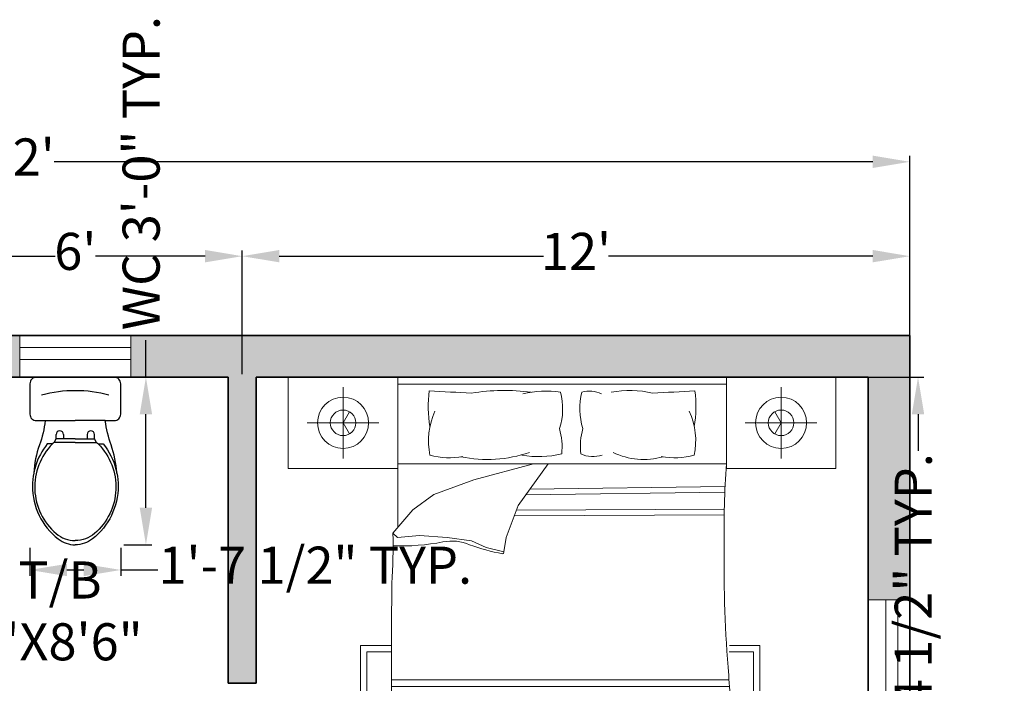
# Model space of a CAD drawing. Units: inches. Extents: x 2073 to 2646, y 2372 to 3017.
# Tile 8 of 8: x 2340 to 2553, y 2874 to 3017. Entities that reach past the tile are written whole.
import ezdxf

# ---------------------------------------------------------------- set-up
doc = ezdxf.new("R2010")
doc.units = ezdxf.units.IN
for name, color, linetype, lineweight in [('A-ANNO-DIMS', 2, 'Continuous', 18), ('A-AREA-IDEN', 7, 'Continuous', 25), ('A-FLOR-FIXT', 9, 'Continuous', 18), ('A-FURN', 8, 'Continuous', 18), ('A-GLAZ', 4, 'Continuous', 18), ('A-WALL', 7, 'Continuous', 35), ('A-WALL-PATT', 30, 'Continuous', 13)]:
    doc.layers.add(name, color=color, linetype=linetype, lineweight=lineweight)
doc.layers.add('WC-Detail_dwgmodels.com', color=251, linetype='Continuous')
doc.layers.add('WC-Outline_dwgmodels.com', color=250, linetype='Continuous')
doc.styles.get("Standard").update_dxf_attribs({"font": 'arial.ttf'})
doc.dimstyles.new('ISO-25', dxfattribs={"dimtxt": 8, "dimasz": 8, "dimexe": 1.25, "dimexo": 0.625, "dimtad": 0, "dimdec": 1, "dimlunit": 4, "dimtxsty": 'Standard', "dimcen": 2.5, "dimadec": 0, "dimazin": 0, "dimtfac": 1, "dimtdec": 1, "dimtmove": 0, "dimatfit": 3, "dimfxl": 1, "dimarcsym": 0})

# ---------------------------------------------------------------- blocks, each defined once
blk = doc.blocks.new('*D5')
at = {"layer": 'A-ANNO-DIMS', "color": 0, "lineweight": -2, "transparency": 16777216}
for p, q in [((2316.29, 2940.29), (2316.29, 2967.03)), ((2388.29, 2940.29), (2388.29, 2967.03)), ((2324.29, 2965.78), (2347.96, 2965.78)), ((2380.29, 2965.78), (2356.62, 2965.78))]:
    blk.add_line(p, q, dxfattribs=at)
at = {"layer": 'A-ANNO-DIMS', "color": 0, "transparency": 16777216}
for points in [[(2324.29, 2967.12), (2324.29, 2964.45), (2316.29, 2965.78)], [(2380.29, 2967.12), (2380.29, 2964.45), (2388.29, 2965.78)]]:
    blk.add_solid(points, dxfattribs=at)
at = {"layer": 'Defpoints', "color": 0, "transparency": 16777216}
for p in [(2388.29, 2965.78), (2316.29, 2939.66), (2388.29, 2939.66)]:
    blk.add_point(p, dxfattribs=at)
at = {"layer": 'A-ANNO-DIMS', "color": 0, "transparency": 16777216, "insert": (2352.29, 2965.78), "char_height": 8, "attachment_point": 5}
blk.add_mtext("6'", dxfattribs=at)
blk = doc.blocks.new('*D6')
at = {"layer": 'A-ANNO-DIMS', "color": 0, "lineweight": -2, "transparency": 16777216}
for p, q in [((2388.29, 2940.29), (2388.29, 2967.03)), ((2532.29, 2940.29), (2532.29, 2967.03)), ((2396.29, 2965.78), (2453.25, 2965.78)), ((2524.29, 2965.78), (2467.33, 2965.78))]:
    blk.add_line(p, q, dxfattribs=at)
at = {"layer": 'A-ANNO-DIMS', "color": 0, "transparency": 16777216}
for points in [[(2396.29, 2967.12), (2396.29, 2964.45), (2388.29, 2965.78)], [(2524.29, 2967.12), (2524.29, 2964.45), (2532.29, 2965.78)]]:
    blk.add_solid(points, dxfattribs=at)
at = {"layer": 'Defpoints', "color": 0, "transparency": 16777216}
for p in [(2532.29, 2965.78), (2388.29, 2939.66), (2532.29, 2939.66)]:
    blk.add_point(p, dxfattribs=at)
at = {"layer": 'A-ANNO-DIMS', "color": 0, "transparency": 16777216, "insert": (2460.29, 2965.78), "char_height": 8, "attachment_point": 5}
blk.add_mtext("12'", dxfattribs=at)
blk = doc.blocks.new('*D7')
at = {"layer": 'A-ANNO-DIMS', "color": 0, "lineweight": -2, "transparency": 16777216}
for p, q in [((2148.29, 2949.29), (2148.29, 2987.4)), ((2156.29, 2986.15), (2332.88, 2986.15)), ((2524.29, 2986.15), (2347.7, 2986.15)), ((2532.29, 2950.58), (2532.29, 2987.4))]:
    blk.add_line(p, q, dxfattribs=at)
at = {"layer": 'A-ANNO-DIMS', "color": 0, "transparency": 16777216}
for points in [[(2156.29, 2987.48), (2156.29, 2984.81), (2148.29, 2986.15)], [(2524.29, 2987.48), (2524.29, 2984.81), (2532.29, 2986.15)]]:
    blk.add_solid(points, dxfattribs=at)
at = {"layer": 'Defpoints', "color": 0, "transparency": 16777216}
for p in [(2148.29, 2986.15), (2148.29, 2948.66), (2532.29, 2949.95)]:
    blk.add_point(p, dxfattribs=at)
at = {"layer": 'A-ANNO-DIMS', "color": 0, "transparency": 16777216, "insert": (2340.29, 2986.15), "char_height": 8, "attachment_point": 5}
blk.add_mtext("32'", dxfattribs=at)
blk = doc.blocks.new('pan')
at = {"layer": 'WC-Detail_dwgmodels.com'}
for p, q in [((2373.08, 3021.25), (2373.44, 3021.91)), ((2373.44, 3021.91), (2373.44, 3022.64)), ((2374.73, 3021.91), (2373.44, 3021.91)), ((2374.73, 3022.64), (2374.73, 3021.91)), ((2376.79, 3021.91), (2374.73, 3021.91)), ((2376.79, 3021.91), (2378.86, 3021.91)), ((2378.86, 3022.64), (2378.86, 3021.91)), ((2378.86, 3021.91), (2380.15, 3021.91)), ((2380.15, 3021.91), (2380.15, 3022.64)), ((2380.51, 3021.25), (2380.15, 3021.91))]:
    blk.add_line(p, q, dxfattribs=at)
for points in [[(2372.8, 3020.99, 0.434217), (2373.44, 3005.35, 0.182634), (2376.79, 3004.12, 2.693815)], [(2371.91, 3020.99, 0.094048), (2369.85, 3017.12, 0.16845)], [(2372.8, 3020.99), (2371.91, 3020.99, 0.416606)], [(2373.08, 3021.25, 0.008985), (2372.8, 3020.99, 0.182634)], [(2376.79, 3021.25), (2373.08, 3021.25, 0.008985)], [(2376.79, 3021.25), (2380.51, 3021.25, -0.444938)], [(2380.79, 3020.99, -0.434217), (2380.15, 3005.35, -0.182634), (2376.79, 3004.12, -2.693815)], [(2380.51, 3021.25, -0.008985), (2380.79, 3020.99, -0.182634)], [(2380.79, 3020.99), (2381.68, 3020.99, -0.416606)], [(2381.68, 3020.99, -0.105447), (2383.88, 3016.61, -0.16845)], [(2369.85, 3017.12, 0.026594), (2369.55, 3015.91, 0.16845)], [(2383.88, 3016.61, -0.015301), (2384.04, 3015.91, -0.16845)]]:
    blk.add_lwpolyline(points, format="xyb", dxfattribs=at)
for centre, radius, start, end in [((2376.81, 3007.03), 23.26, 90.028, 104.6712), ((2376.78, 3007.03), 23.26, 75.3288, 89.972), ((2374.08, 3022.64), 0.645, 0, 180), ((2379.51, 3022.64), 0.645, 0, 180)]:
    blk.add_arc(centre, radius, start, end, dxfattribs=at)
at = {"layer": 'WC-Outline_dwgmodels.com'}
for points in [[(2383.59, 3025.06, 0.414214), (2384.72, 3026.19), (2384.72, 3031.5, 0.414214), (2383.59, 3032.64), (2376.79, 3032.64), (2370, 3032.64, 0.414214), (2368.87, 3031.5), (2368.87, 3026.19, 0.414214), (2370, 3025.06), (2371.56, 3025.06, -0.052345), (2370.54, 3020.81, 0.071131), (2369.55, 3015.91, 0.160777)], [(2371.56, 3025.06), (2376.79, 3025.06, 0.414214)], [(2382.03, 3025.06), (2376.79, 3025.06, -0.414214)], [(2384.04, 3015.91, 0.071131), (2383.05, 3020.81, -0.052345), (2382.03, 3025.06), (2383.59, 3025.06, 0.414214)], [(2369.55, 3015.91, 0.048023), (2369.32, 3013.67, 0.16845)], [(2384.04, 3015.91, -0.048023), (2384.27, 3013.67, -0.16845)], [(2369.32, 3013.67, 0.230343), (2373.8, 3004.42, 0.16845), (2376.79, 3003.38, 2.883082)], [(2384.27, 3013.67, -0.230343), (2379.79, 3004.42, -0.16845), (2376.79, 3003.38, -2.883082)]]:
    blk.add_lwpolyline(points, format="xyb", dxfattribs=at)
blk = doc.blocks.new('bed')
at = {"color": 0}
for p, q in [((2249.53, 3172.75), (2367.64, 3172.75)), ((2273.15, 3172.75), (2273.15, 3140.33)), ((2344.02, 3171.23), (2273.15, 3171.23)), ((2261.34, 3155.19), (2261.34, 3170.62)), ((2355.83, 3155.19), (2355.83, 3170.62)), ((2269.06, 3162.9), (2253.62, 3162.9)), ((2348.11, 3162.9), (2363.55, 3162.9)), ((2273.15, 3154.08), (2344.02, 3154.08)), ((2289.56, 3150.57), (2302.44, 3154.08)), ((2305.6, 3154.08), (2299.13, 3145.07)), ((2280.95, 3147.46), (2289.56, 3150.57)), ((2343.66, 3147.96), (2300.77, 3147.36)), ((2343.7, 3149.18), (2301.65, 3148.59)), ((2276.4, 3144.12), (2280.95, 3147.46)), ((2272.09, 3139.1), (2276.4, 3144.12)), ((2299.13, 3145.07), (2296.5, 3138.14)), ((2343.59, 3144.24), (2298.75, 3144.07)), ((2343.6, 3143.03), (2298.28, 3142.85)), ((2273.05, 3138.14), (2272.09, 3139.1)), ((2277.84, 3138.62), (2273.05, 3138.14)), ((2283.82, 3138.14), (2277.84, 3138.62)), ((2289.08, 3137.42), (2283.82, 3138.14)), ((2292.19, 3135.99), (2289.08, 3137.42)), ((2296.5, 3138.14), (2296.02, 3135.03)), ((2296.02, 3135.03), (2292.19, 3135.99)), ((2265.12, 3114.85), (2271.8, 3114.85)), ((2265.12, 3072.3), (2265.12, 3114.85)), ((2344.68, 3114.85), (2351.23, 3114.85)), ((2351.23, 3114.85), (2351.23, 3072.3)), ((2271.8, 3113.48), (2266.49, 3113.48)), ((2266.49, 3113.48), (2266.49, 3073.67)), ((2349.86, 3113.48), (2344.65, 3113.48)), ((2349.86, 3073.67), (2349.86, 3113.48)), ((2344.56, 3107.48), (2271.79, 3107.48)), ((2344.67, 3106.01), (2271.79, 3106.01)), ((2332.56, 3094.41), (2284.61, 3094.41)), ((2278.13, 3085.65), (2277.87, 3086.98)), ((2286.38, 3085.65), (2286.64, 3086.98)), ((2329.96, 3085.65), (2329.7, 3086.98)), ((2338.22, 3085.65), (2338.48, 3086.98)), ((2266.49, 3073.67), (2349.86, 3073.67)), ((2351.23, 3072.3), (2265.12, 3072.3))]:
    blk.add_line(p, q, dxfattribs=at)
for points in [[(2273.15, 3153.06), (2249.53, 3153.06), (2249.53, 3172.75)], [(2344.02, 3172.75), (2344.02, 3153.06), (2367.64, 3153.06), (2367.64, 3172.75)], [(2261.34, 3162.9), (2262.72, 3165.29)], [(2355.83, 3162.9), (2354.45, 3165.29)], [(2261.34, 3162.9), (2262.72, 3160.52)], [(2355.83, 3162.9), (2354.45, 3160.52)]]:
    blk.add_lwpolyline(points, dxfattribs=at)
for points in [[(2279.94, 3169.8, 0.074897), (2280.08, 3162.09, -0.472817)], [(2308.03, 3161.66, 0.14099), (2308.27, 3169.53, 0.235245)], [(2313.08, 3161.66, -0.14099), (2312.84, 3169.53, -0.235245)], [(2337.23, 3169.8, -0.074897), (2337.09, 3162.09, 0.472817)], [(2271.85, 3128.28, 0.001242), (2271.79, 3105.87, -0.127202), (2269.42, 3094.7)], [(2344.52, 3108.41, 0.056112), (2345.38, 3101.91, 0.095341), (2347.04, 3095.66)]]:
    blk.add_lwpolyline(points, format="xyb", dxfattribs=at)
for centre, radius in [((2261.34, 3162.9), 5.51), ((2355.83, 3162.9), 5.51), ((2261.34, 3162.9), 2.76), ((2355.83, 3162.9), 2.76), ((2284.95, 3081.37), 0.301), ((2331.4, 3081.37), 0.301), ((2282.98, 3078.2), 0.301), ((2333.36, 3078.2), 0.301)]:
    blk.add_circle(centre, radius, dxfattribs=at)
for centre, radius, start, end in [((2345.04, 4293.82), 1125.9, 266.68521, 267.14978), ((2296.12, 3127.06), 42.84, 82.2196, 99.497), ((2305.17, 3148.71), 21.05, 81.5249, 103.96), ((2314.46, 3163.91), 5.84, 63.3437, 106.1026), ((2323.22, 3149.14), 20.76, 76.3427, 101.1841), ((2272.13, 4293.82), 1125.9, 272.85022, 273.31479), ((2294.98, 3158.99), 15.22, 155.1316, 191.7583), ((2322.19, 3158.99), 15.22, 348.2417, 24.8684), ((2294.11, 3157.71), 14.47, 354.0129, 15.8293), ((2327, 3157.71), 14.47, 164.1707, 185.9871), ((2292.48, 3182.44), 27.45, 258.0397, 289.2615), ((2303.6, 3176.44), 20.83, 259.8617, 283.6238), ((2315.25, 3161.88), 6.26, 245.0183, 288.5407), ((2326.19, 3170.02), 15.03, 243.8761, 286.1746), ((2284.15, 3171.19), 15.83, 255.1039, 281.0369), ((2333.02, 3171.19), 15.83, 258.9631, 284.8961), ((2555.75, 3139.65), 212.22, 176.1, 180.9282), ((2163.8, 3136.16), 108.33, 355.8294, 1.553), ((2274.12, 3180.92), 44.58, 267.4519, 281.3392), ((2284.77, 3127.79), 9.61, 66.2616, 101.3392), ((2304.22, 3179.66), 45.8, 250.1194, 259.3383), ((2295.75, 3134.94), 0.285, 268.8623, 19.7536), ((2620.36, 3131.93), 276.84, 179.1145, 184.8735), ((2270.51, 3094.78), 1.09, 183.98, 297.3412), ((2283.2, 2971.46), 122.95, 89.3433, 95.6887), ((2285.12, 3093.1), 1.42, 113.229, 135.5483), ((2285.12, 3093.1), 1.42, 37.675, 66.7144), ((2291.18, 3093.53), 4.89, 169.7133, 211.1782), ((2294.46, 3086.09), 8.94, 111.4941, 146.3329), ((2321.89, 3086.09), 8.94, 33.6671, 68.5059), ((2325.17, 3093.53), 4.89, 328.8218, 10.2867), ((2331.23, 3093.1), 1.42, 113.2856, 142.325), ((2331.23, 3093.1), 1.42, 44.4517, 66.7144), ((2336.18, 2979.53), 114.93, 85.2402, 91.8035), ((2336.96, 3093.1), 1.42, 106.6343, 135.5483), ((2336.96, 3093.1), 1.42, 37.675, 72.5814), ((2343.02, 3093.53), 4.89, 169.249, 211.1782), ((2346.15, 3095.06), 1.08, 246.5219, 33.8264), ((2275.26, 3090.38), 1.99, 84.4856, 181.0538), ((2270.05, 3086.09), 8.94, 33.6671, 63.2997), ((2274.65, 3088.91), 3.55, 355.2933, 76.921), ((2282.03, 3091.41), 4.56, 145.785, 184.7304), ((2273.33, 3093.53), 4.89, 328.8218, 9.1554), ((2279.39, 3093.1), 1.42, 120.0293, 142.325), ((2277.12, 3092.26), 3.76, 289.2822, 29.1751), ((2276.55, 3091.58), 3.4, 7.436, 29.9149), ((2278.79, 3093.38), 1.77, 311.5653, 23.8354), ((2279.39, 3093.1), 1.42, 44.4517, 63.558), ((2287.39, 3092.26), 3.76, 150.8249, 250.7178), ((2285.72, 3093.38), 1.77, 156.1646, 228.4347), ((2287.96, 3091.58), 3.4, 150.0851, 172.564), ((2282.48, 3091.41), 4.56, 355.2696, 34.215), ((2289.86, 3088.91), 3.55, 103.079, 184.7067), ((2289.25, 3090.38), 1.99, 358.9462, 95.5144), ((2327.09, 3090.38), 1.99, 84.4856, 181.0538), ((2326.48, 3088.91), 3.55, 355.2933, 76.921), ((2333.87, 3091.41), 4.56, 145.785, 184.7304), ((2328.96, 3092.26), 3.76, 289.2822, 29.1751), ((2328.39, 3091.58), 3.4, 7.436, 29.9149), ((2330.63, 3093.38), 1.77, 311.5653, 23.8354), ((2339.23, 3092.26), 3.76, 150.8249, 250.7178), ((2337.56, 3093.38), 1.77, 156.1646, 228.4347), ((2339.8, 3091.58), 3.4, 150.0851, 172.564), ((2334.32, 3091.41), 4.56, 355.2696, 34.215), ((2341.7, 3088.91), 3.55, 103.079, 184.7067), ((2346.3, 3086.09), 8.94, 113.6453, 146.3329), ((2341.09, 3090.38), 1.99, 358.9462, 95.5144), ((2276.08, 3090.1), 2.82, 174.9449, 262.8857), ((2277.18, 3091.17), 2.74, 201.5819, 291.4221), ((2276.66, 3088.19), 2.94, 299.9085, 73.1337), ((2281.57, 3090.25), 2.42, 131.5653, 195.1471), ((2282.94, 3090.25), 2.42, 344.8529, 48.4347), ((2287.85, 3088.19), 2.94, 106.8663, 240.0915), ((2287.32, 3091.17), 2.74, 248.5779, 338.4181), ((2288.43, 3090.1), 2.82, 277.1143, 5.0551), ((2327.91, 3090.1), 2.82, 174.9449, 262.8857), ((2329.02, 3091.17), 2.74, 201.5819, 291.4221), ((2328.5, 3088.19), 2.94, 299.9085, 73.1337), ((2333.4, 3090.25), 2.42, 131.5653, 195.1471), ((2334.78, 3090.25), 2.42, 344.8529, 48.4347), ((2339.68, 3088.19), 2.94, 106.8663, 240.0915), ((2339.16, 3091.17), 2.74, 248.5779, 338.4181), ((2340.27, 3090.1), 2.82, 277.1143, 5.0551), ((2275.58, 3090.72), 3.43, 272.3591, 324.0401), ((2271.86, 3089), 6.34, 326.2883, 356.5076), ((2282.03, 3091.41), 4.56, 212.7011, 216.3445), ((2278.52, 3089.43), 0.733, 257.3041, 15.1471), ((2282.59, 3088.31), 0.228, 102.7051, 280.4384), ((2282.57, 3088.45), 0.37, 280.4384, 100.4136), ((2285.99, 3089.43), 0.733, 164.8529, 282.6959), ((2282.48, 3091.41), 4.56, 323.6555, 327.2989), ((2288.92, 3090.72), 3.43, 215.9599, 267.6409), ((2292.65, 3089), 6.34, 183.4924, 213.7117), ((2327.42, 3090.72), 3.43, 272.3591, 324.0401), ((2323.7, 3089), 6.34, 326.2883, 356.5076), ((2333.87, 3091.41), 4.56, 212.7011, 216.3445), ((2330.36, 3089.43), 0.733, 257.3041, 15.1471), ((2333.78, 3088.45), 0.37, 79.5864, 259.5616), ((2333.75, 3088.31), 0.228, 259.5616, 77.2949), ((2337.82, 3089.43), 0.733, 164.8529, 282.6959), ((2334.32, 3091.41), 4.56, 323.6555, 327.2989), ((2340.76, 3090.72), 3.43, 215.9599, 267.6409), ((2344.49, 3089), 6.34, 183.4924, 213.7117), ((2275.43, 3085.55), 1.77, 80.264, 250.8688), ((2271.91, 3089.45), 5.58, 301.2614, 341.7045), ((2290.78, 3082.37), 9.78, 153.0032, 159.8941), ((2281.96, 3085.71), 0.241, 84.3784, 186.0543), ((2281.48, 3087.78), 1.9, 285.5129, 293.6099), ((2282.72, 3085.65), 0.62, 87.3579, 140.4944), ((2281.28, 3087.43), 1.87, 301.164, 321.5612), ((2279.77, 3087.76), 3.33, 324.6898, 333.4936), ((2292.6, 3089.45), 5.58, 198.2955, 238.7386), ((2289.08, 3085.55), 1.77, 289.1312, 99.736), ((2309.5, 3071.59), 15.42, 94.4623, 172.255), ((2309.57, 3085.82), 1.71, 137.7873, 219.1145), ((2307.63, 3085.87), 1.29, 298.5391, 58.3627), ((2309.53, 3086.61), 1.28, 63.0274, 163.8037), ((2308.24, 3089.6), 2.63, 271.4585, 315.3727), ((2309.31, 3084.75), 2.44, 45.5411, 114.3101), ((2311.53, 3097.27), 10.79, 252.593, 267.2582), ((2309.56, 3086.92), 1.26, 177.7585, 283.852), ((2311.99, 3088.23), 3.9, 198.9159, 238.011), ((2310.98, 3084.75), 2.44, 65.6899, 134.4589), ((2308.75, 3097.27), 10.79, 272.7418, 287.407), ((2309.83, 3085.86), 0.167, 283.852, 219.9245), ((2310.75, 3086.61), 1.28, 16.1963, 116.9726), ((2312.05, 3089.6), 2.63, 224.6273, 268.5415), ((2310.44, 3085.92), 0.101, 320.1909, 256.0209), ((2308.29, 3088.23), 3.9, 301.989, 341.0841), ((2310.72, 3086.92), 1.26, 256.148, 2.2415), ((2312.66, 3085.87), 1.29, 121.6373, 241.4609), ((2310.71, 3085.82), 1.71, 320.8855, 42.2127), ((2310.28, 3075.15), 11.94, 352.8636, 81.8197), ((2327.26, 3085.55), 1.77, 80.264, 250.8688), ((2323.75, 3089.45), 5.58, 301.2614, 341.7045), ((2335.06, 3087.43), 1.87, 218.4388, 238.836), ((2333.63, 3085.65), 0.62, 39.5056, 92.6421), ((2336.58, 3087.76), 3.33, 206.5064, 215.3102), ((2334.87, 3087.78), 1.9, 246.3901, 254.4871), ((2325.57, 3082.37), 9.78, 20.1059, 26.9968), ((2334.38, 3085.71), 0.241, 353.9457, 95.6216), ((2344.44, 3089.45), 5.58, 198.2955, 238.7386), ((2340.92, 3085.55), 1.77, 289.1312, 99.736), ((2273.92, 3083.1), 1.28, 92.9516, 193.728), ((2271.31, 3085.04), 2.63, 301.3827, 345.2969), ((2274.66, 3081.37), 2.44, 75.4653, 144.2343), ((2275.06, 3083.63), 1.09, 63.9755, 143.2681), ((2275, 3086.08), 2.21, 265.969, 344.3045), ((2277.38, 3083.14), 2.36, 96.1662, 141.5825), ((2279.54, 3083.62), 0.502, 101.5637, 142.6358), ((2279.13, 3084.01), 0.723, 288.7263, 352.5032), ((2279.63, 3083.98), 0.232, 345.2356, 144.9248), ((2281.29, 3084.79), 0.62, 101.3256, 154.4621), ((2280.4, 3086.9), 1.87, 280.2588, 300.656), ((2280.83, 3088.39), 3.33, 268.3264, 277.1302), ((2290.78, 3082.37), 9.78, 163.5842, 183.8277), ((2279.99, 3086.89), 1.9, 308.2101, 316.3071), ((2281.16, 3085.65), 0.567, 278.3432, 4.2869), ((2280.84, 3086.14), 0.99, 300.656, 332.6341), ((2281.59, 3085.49), 0.241, 55.7657, 157.4417), ((2281.74, 3086.68), 0.99, 269.1859, 301.164), ((2282.03, 3086.17), 0.567, 237.5332, 323.4768), ((2287.12, 3083.14), 2.36, 38.4175, 83.8338), ((2289.51, 3086.08), 2.21, 195.6955, 274.031), ((2289.45, 3083.63), 1.09, 36.7319, 116.0245), ((2289.85, 3081.37), 2.44, 35.7657, 104.5347), ((2290.59, 3083.1), 1.28, 346.272, 87.0484), ((2293.2, 3085.04), 2.63, 194.7031, 238.6173), ((2310.03, 3085.09), 0.192, 238.011, 71.5592), ((2310.06, 3085.18), 0.093, 71.5592, 188.0167), ((2310.25, 3085.09), 0.192, 108.4408, 301.989), ((2310.22, 3085.18), 0.093, 351.9833, 108.4408), ((2325.76, 3083.1), 1.28, 92.9516, 193.728), ((2323.15, 3085.04), 2.63, 301.3827, 345.2969), ((2326.5, 3081.37), 2.44, 75.4653, 144.2343), ((2326.9, 3083.63), 1.09, 63.9755, 143.2681), ((2326.84, 3086.08), 2.21, 265.969, 344.3045), ((2329.22, 3083.14), 2.36, 96.1662, 141.5825), ((2334.32, 3086.17), 0.567, 216.5232, 302.4668), ((2334.61, 3086.68), 0.99, 238.836, 270.8141), ((2334.76, 3085.49), 0.241, 22.5583, 124.2343), ((2335.19, 3085.65), 0.567, 175.7131, 261.6568), ((2335.5, 3086.14), 0.99, 207.3659, 239.344), ((2325.57, 3082.37), 9.78, 356.1723, 16.4158), ((2336.35, 3086.89), 1.9, 223.6929, 231.7899), ((2335.95, 3086.9), 1.87, 239.344, 259.7412), ((2335.52, 3088.39), 3.33, 262.8698, 271.6736), ((2335.06, 3084.79), 0.62, 25.5379, 78.6744), ((2336.72, 3083.98), 0.232, 35.0752, 194.7644), ((2337.21, 3084.01), 0.723, 187.4968, 251.2737), ((2336.81, 3083.62), 0.502, 37.3642, 78.4363), ((2341.35, 3086.08), 2.21, 195.6955, 274.031), ((2338.96, 3083.14), 2.36, 38.4175, 83.8338), ((2341.29, 3083.63), 1.09, 36.7319, 116.0245), ((2341.69, 3081.37), 2.44, 35.7657, 104.5347), ((2345.04, 3085.04), 2.63, 194.7031, 238.6173), ((2342.42, 3083.1), 1.28, 346.272, 87.0484), ((2255.01, 3071.59), 15.42, 7.745, 41.8856), ((2281.39, 3070.07), 15.42, 124.3865, 158.5908), ((2274.35, 3082.43), 1.71, 167.7115, 249.0387), ((2270.34, 3093.33), 10.79, 282.5173, 297.1824), ((2272.64, 3081.51), 1.29, 328.4633, 88.2869), ((2275.25, 3085.73), 3.9, 228.8402, 267.9352), ((2273.8, 3083.38), 1.26, 207.6827, 313.7762), ((2274.56, 3082.59), 0.167, 313.7762, 249.7183), ((2275.1, 3082.12), 0.093, 101.4834, 217.9409), ((2275.12, 3082.03), 0.192, 267.9352, 101.4834), ((2279.12, 3083.15), 0.301, 273.2768, 86.7232), ((2279.53, 3082.6), 0.497, 217.7621, 259.0403), ((2279.47, 3083.44), 0.287, 91.1081, 181.8675), ((2280.07, 3083.26), 0.913, 203.4276, 227.6104), ((2279.78, 3082.86), 0.622, 80.3487, 133.6538), ((2279.66, 3083.37), 0.492, 229.7889, 317.6792), ((2279.11, 3082.33), 0.699, 355.053, 68.3618), ((2279.66, 3082.21), 0.985, 83.0852, 105.7171), ((2279.58, 3082.29), 0.231, 232.4737, 355.053), ((2272.84, 3074.04), 11.21, 43.1541, 52.0459), ((2279.84, 3083.22), 0.259, 317.6792, 80.3487), ((2280.45, 3081.67), 0.567, 278.3432, 4.2869), ((2280.14, 3082.17), 0.99, 300.656, 332.6341), ((2280.88, 3081.52), 0.241, 55.7657, 157.4417), ((2285.91, 3082.12), 4.9, 184.756, 209.2041), ((2292.97, 3092.56), 16.14, 222.2412, 232.1744), ((2282.65, 3081.81), 1.37, 304.5369, 16.3699), ((2284.55, 3081.43), 0.97, 127.3105, 187.9252), ((2283.22, 3081.54), 0.996, 355.0106, 41.658), ((2284.62, 3081.78), 0.41, 126.1046, 271.4281), ((2284.57, 3081.9), 0.295, 353.7526, 131.7054), ((2284.3, 3081.55), 0.414, 0.0645, 61.1507), ((2284.39, 3081.9), 0.473, 311.8413, 355.7877), ((2285.37, 3081.83), 0.502, 101.5637, 176.365), ((2285.3, 3081.65), 0.287, 91.1081, 181.8675), ((2285.61, 3081.07), 0.622, 80.3487, 133.6538), ((2284.96, 3082.22), 0.723, 288.7263, 352.5032), ((2285.46, 3082.19), 0.232, 345.2356, 144.9248), ((2285.67, 3081.43), 0.259, 317.6792, 80.3487), ((2289.39, 3082.03), 0.192, 78.5166, 272.0648), ((2294.17, 3093.33), 10.79, 242.8176, 257.4827), ((2289.26, 3085.73), 3.9, 272.0648, 311.1598), ((2289.41, 3082.12), 0.093, 322.0591, 78.5166), ((2290.71, 3083.38), 1.26, 226.2238, 332.3173), ((2289.97, 3082.66), 0.101, 290.2667, 226.2271), ((2291.87, 3081.51), 1.29, 91.7131, 211.5367), ((2290.16, 3082.43), 1.71, 290.9613, 12.2885), ((2283.12, 3070.07), 15.42, 21.4092, 55.6135), ((2333.23, 3070.07), 15.42, 124.3865, 158.5908), ((2326.19, 3082.43), 1.71, 167.7115, 249.0387), ((2322.18, 3093.33), 10.79, 282.5173, 297.1824), ((2325.64, 3083.38), 1.26, 207.6827, 313.7762), ((2327.09, 3085.73), 3.9, 228.8402, 267.9352), ((2324.48, 3081.51), 1.29, 328.4633, 88.2869), ((2326.39, 3082.59), 0.167, 313.7762, 249.7183), ((2326.93, 3082.12), 0.093, 101.4834, 217.9409), ((2326.95, 3082.03), 0.192, 267.9352, 101.4834), ((2330.68, 3081.43), 0.259, 99.6513, 222.3208), ((2330.74, 3081.07), 0.622, 46.3462, 99.6513), ((2330.89, 3082.19), 0.232, 35.0752, 194.7644), ((2331.38, 3082.22), 0.723, 187.4968, 251.2737), ((2331.05, 3081.65), 0.287, 358.1325, 88.8919), ((2330.98, 3081.83), 0.502, 3.635, 78.4363), ((2331.77, 3081.9), 0.295, 48.2946, 186.2474), ((2331.95, 3081.9), 0.473, 184.2123, 228.1587), ((2332.05, 3081.55), 0.414, 118.8493, 179.9355), ((2331.73, 3081.78), 0.41, 268.5719, 53.8954), ((2333.13, 3081.54), 0.996, 138.342, 184.9894), ((2333.7, 3081.81), 1.37, 163.6301, 235.4631), ((2331.79, 3081.43), 0.97, 352.0748, 52.6895), ((2323.38, 3092.56), 16.14, 307.8256, 317.7588), ((2330.44, 3082.12), 4.9, 330.7959, 355.244), ((2343.51, 3074.04), 11.21, 127.9541, 136.8459), ((2335.46, 3081.52), 0.241, 22.5583, 124.2343), ((2335.89, 3081.67), 0.567, 175.7131, 261.6568), ((2336.21, 3082.17), 0.99, 207.3659, 239.344), ((2336.51, 3083.22), 0.259, 99.6513, 222.3208), ((2336.68, 3083.37), 0.492, 222.3208, 310.2111), ((2336.57, 3082.86), 0.622, 46.3462, 99.6513), ((2337.24, 3082.33), 0.699, 111.6382, 184.947), ((2336.77, 3082.29), 0.231, 184.947, 307.5263), ((2336.69, 3082.21), 0.985, 74.2829, 96.9148), ((2336.88, 3083.44), 0.287, 358.1325, 88.8919), ((2336.28, 3083.26), 0.913, 312.3896, 336.5724), ((2336.82, 3082.6), 0.497, 280.9597, 322.2379), ((2337.23, 3083.15), 0.301, 93.2768, 266.7232), ((2341.23, 3082.03), 0.192, 78.5166, 272.0648), ((2346, 3093.33), 10.79, 242.8176, 257.4827), ((2341.1, 3085.73), 3.9, 272.0648, 311.1598), ((2341.25, 3082.12), 0.093, 322.0591, 78.5166), ((2342.55, 3083.38), 1.26, 226.2238, 332.3173), ((2341.81, 3082.66), 0.101, 290.2667, 226.2271), ((2343.7, 3081.51), 1.29, 91.7131, 211.5367), ((2341.99, 3082.43), 1.71, 290.9613, 12.2885), ((2334.95, 3070.07), 15.42, 21.4092, 55.6135), ((2361.34, 3071.59), 15.42, 138.1144, 172.255), ((2280.59, 3080.82), 0.62, 101.3256, 154.4621), ((2279.69, 3082.92), 1.87, 280.2588, 300.656), ((2280.12, 3084.42), 3.33, 268.3264, 277.1302), ((2279.29, 3082.92), 1.9, 308.2101, 316.3071), ((2280.79, 3079.73), 0.336, 146.8636, 236.9021), ((2285.53, 3087.13), 8.79, 235.1882, 238.8844), ((2281.37, 3080.22), 0.909, 199.4799, 267.6828), ((2281.17, 3079.91), 0.348, 238.8844, 314.2646), ((2281.59, 3079.27), 0.262, 19.3605, 201.7548), ((2281.59, 3079.47), 0.262, 311.8703, 134.2646), ((2282.36, 3080.66), 1.37, 247.2305, 319.0635), ((2281.9, 3080.2), 0.807, 264.4544, 310.6188), ((2286.41, 3075.61), 5.88, 120.544, 139.818), ((2283.06, 3078.85), 0.97, 70.0041, 130.6188), ((2282.43, 3080.03), 0.996, 297.7043, 344.3516), ((2283.38, 3081.51), 0.833, 272.8499, 356.1226), ((2282.79, 3081.18), 0.807, 321.7607, 7.9252), ((2282.96, 3080.02), 0.807, 8.7227, 54.8872), ((2283, 3079.38), 1.37, 0.278, 72.111), ((2283.62, 3079.88), 0.833, 20.5253, 88.5375), ((2284.72, 3080.29), 0.97, 188.7227, 249.3375), ((2284.32, 3080.8), 0.298, 148.0499, 225.6268), ((2286.41, 3075.61), 5.88, 113.0501, 113.8477), ((2284.87, 3080.46), 0.948, 104.7558, 148.0499), ((2284.34, 3081.14), 0.594, 247.4086, 351.4386), ((2283.47, 3079.81), 0.996, 334.9899, 21.6373), ((2284.51, 3081.11), 0.199, 262.906, 7.132), ((2285.36, 3080.81), 0.497, 151.2196, 259.0403), ((2285.9, 3081.47), 0.913, 203.4276, 227.6104), ((2285.5, 3081.59), 0.492, 229.7889, 317.6792), ((2284.94, 3080.54), 0.699, 355.053, 68.3618), ((2285.49, 3080.43), 0.985, 83.0852, 105.7171), ((2285.41, 3080.5), 0.231, 232.4737, 355.053), ((2286.41, 3075.61), 5.88, 87.1071, 94.7585), ((2308.35, 3078.35), 1.28, 63.0274, 163.8037), ((2311.93, 3078.35), 1.28, 16.1963, 116.9726), ((2329.94, 3075.61), 5.88, 85.2415, 92.8929), ((2330.85, 3081.59), 0.492, 222.3208, 310.2111), ((2331.41, 3080.54), 0.699, 111.6382, 184.947), ((2330.94, 3080.5), 0.231, 184.947, 307.5263), ((2330.86, 3080.43), 0.985, 74.2829, 96.9148), ((2330.45, 3081.47), 0.913, 312.3896, 336.5724), ((2330.99, 3080.81), 0.497, 280.9597, 28.7804), ((2332.01, 3081.14), 0.594, 188.5614, 292.5914), ((2331.84, 3081.11), 0.199, 172.868, 277.094), ((2331.48, 3080.46), 0.948, 31.9501, 75.2442), ((2332.87, 3079.81), 0.996, 158.3627, 205.0101), ((2332.73, 3079.88), 0.833, 91.4625, 159.4747), ((2333.34, 3079.38), 1.37, 107.889, 179.722), ((2331.63, 3080.29), 0.97, 290.6625, 351.2773), ((2332.97, 3081.51), 0.833, 183.8774, 267.1501), ((2329.94, 3075.61), 5.88, 66.1523, 66.9499), ((2332.03, 3080.8), 0.298, 314.3732, 31.9501), ((2333.39, 3080.02), 0.807, 125.1128, 171.2773), ((2333.55, 3081.18), 0.807, 172.0748, 218.2393), ((2329.94, 3075.61), 5.88, 40.182, 59.456), ((2333.29, 3078.85), 0.97, 49.3812, 109.9959), ((2333.99, 3080.66), 1.37, 220.9365, 292.7695), ((2333.91, 3080.03), 0.996, 195.6484, 242.2957), ((2334.44, 3080.2), 0.807, 229.3812, 275.5456), ((2334.75, 3079.47), 0.262, 45.7354, 228.1297), ((2334.75, 3079.27), 0.262, 338.2452, 160.6395), ((2335.18, 3079.91), 0.348, 225.7354, 301.1156), ((2334.98, 3080.22), 0.909, 272.3172, 340.5201), ((2330.82, 3087.13), 8.79, 301.1156, 304.8118), ((2337.06, 3082.92), 1.9, 223.6929, 231.7899), ((2336.65, 3082.92), 1.87, 239.344, 259.7412), ((2335.55, 3079.73), 0.336, 303.0979, 33.1364), ((2336.22, 3084.42), 3.33, 262.8698, 271.6736), ((2335.76, 3080.82), 0.62, 25.5379, 78.6744), ((2281.27, 3079.88), 0.783, 212.8155, 277.3992), ((2280.81, 3079.35), 0.909, 266.9701, 338.2913), ((2276.02, 3085.84), 8.79, 302.6784, 306.3746), ((2281.04, 3078.63), 0.336, 214.3538, 304.3923), ((2281.09, 3079.13), 0.783, 280.3057, 17.1958), ((2281.03, 3079.05), 0.348, 306.3746, 21.7548), ((2286.53, 3077.08), 5.24, 153.7819, 158.2913), ((2285.91, 3082.12), 4.9, 214.0033, 222.4917), ((2282.49, 3079.88), 0.833, 218.3208, 298.8162), ((2282.35, 3077.63), 0.298, 148.0499, 225.6268), ((2282.9, 3077.29), 0.948, 104.7558, 148.0499), ((2282.37, 3077.97), 0.594, 247.4086, 351.4386), ((2282.65, 3078.61), 0.41, 126.1046, 271.4281), ((2282.61, 3078.72), 0.295, 353.7526, 131.7054), ((2282.54, 3077.94), 0.199, 262.906, 7.132), ((2282.33, 3078.37), 0.414, 0.0645, 61.1507), ((2282.43, 3078.73), 0.473, 311.8413, 355.7877), ((2283.4, 3078.66), 0.502, 101.5637, 176.365), ((2283.39, 3077.64), 0.497, 151.2196, 259.0403), ((2283.33, 3078.48), 0.287, 91.1081, 181.8675), ((2283.93, 3078.3), 0.913, 203.4276, 227.6104), ((2283.64, 3077.9), 0.622, 80.3487, 133.6538), ((2283.53, 3078.42), 0.492, 229.7889, 317.6792), ((2283, 3079.05), 0.723, 288.7263, 352.5032), ((2282.97, 3077.37), 0.699, 355.053, 68.3618), ((2283.52, 3077.26), 0.985, 83.0852, 105.7171), ((2283.49, 3079.02), 0.232, 345.2356, 144.9248), ((2283.7, 3078.26), 0.259, 317.6792, 80.3487), ((2308.32, 3063.33), 15.42, 94.4623, 117.4146), ((2308.39, 3077.56), 1.71, 137.7873, 219.1145), ((2306.45, 3077.61), 1.29, 298.5391, 58.3627), ((2307.06, 3081.34), 2.63, 271.4585, 315.3727), ((2308.13, 3076.49), 2.44, 45.5411, 114.3101), ((2310.81, 3079.97), 3.9, 198.9159, 238.011), ((2310.35, 3089), 10.79, 252.593, 267.2582), ((2308.38, 3078.66), 1.26, 177.7585, 283.852), ((2308.65, 3077.6), 0.167, 283.852, 219.9245), ((2312.16, 3076.49), 2.44, 65.6899, 134.4589), ((2309.93, 3089), 10.79, 272.7418, 287.407), ((2313.23, 3081.34), 2.63, 224.6273, 268.5415), ((2311.62, 3077.66), 0.101, 320.1909, 256.0209), ((2309.47, 3079.97), 3.9, 301.989, 341.0841), ((2311.9, 3078.66), 1.26, 256.148, 2.2415), ((2313.84, 3077.61), 1.29, 121.6373, 241.4609), ((2311.89, 3077.56), 1.71, 320.8855, 42.2127), ((2311.96, 3063.33), 15.42, 62.5854, 85.5377), ((2332.65, 3078.26), 0.259, 99.6513, 222.3208), ((2332.82, 3078.42), 0.492, 222.3208, 310.2111), ((2332.71, 3077.9), 0.622, 46.3462, 99.6513), ((2332.86, 3079.02), 0.232, 35.0752, 194.7644), ((2333.35, 3079.05), 0.723, 187.4968, 251.2737), ((2333.37, 3077.37), 0.699, 111.6382, 184.947), ((2332.83, 3077.26), 0.985, 74.2829, 96.9148), ((2333.01, 3078.48), 0.287, 358.1325, 88.8919), ((2332.42, 3078.3), 0.913, 312.3896, 336.5724), ((2332.95, 3078.66), 0.502, 3.635, 78.4363), ((2332.95, 3077.64), 0.497, 280.9597, 28.7804), ((2333.98, 3077.97), 0.594, 188.5614, 292.5914), ((2333.85, 3079.88), 0.833, 241.1838, 321.6792), ((2333.74, 3078.72), 0.295, 48.2946, 186.2474), ((2333.92, 3078.73), 0.473, 184.2123, 228.1587), ((2334.02, 3078.37), 0.414, 118.8493, 179.9355), ((2333.81, 3077.94), 0.199, 172.868, 277.094), ((2333.7, 3078.61), 0.41, 268.5719, 53.8954), ((2333.44, 3077.29), 0.948, 31.9501, 75.2442), ((2330.44, 3082.12), 4.9, 317.5083, 325.9967), ((2334, 3077.63), 0.298, 314.3732, 31.9501), ((2335.25, 3079.13), 0.783, 162.8042, 259.6943), ((2329.82, 3077.08), 5.24, 21.7087, 26.2181), ((2335.53, 3079.35), 0.909, 201.7087, 273.0299), ((2335.32, 3079.05), 0.348, 158.2452, 233.6254), ((2335.08, 3079.88), 0.783, 262.6008, 327.1845), ((2340.32, 3085.84), 8.79, 233.6254, 237.3216), ((2335.3, 3078.63), 0.336, 235.6077, 325.6462), ((2262.74, 3069.53), 7.52, 33.4617, 60.1116), ((2266.95, 3071.27), 6.27, 22.5547, 48.9546), ((2249.77, 3074.64), 21.34, 357.4081, 3.6519), ((2283.44, 3077.33), 0.231, 232.4737, 355.053), ((2297.56, 3071.27), 6.27, 131.0454, 157.4453), ((2314.73, 3074.64), 21.34, 176.3481, 182.5919), ((2301.77, 3069.53), 7.52, 91.272, 146.5383), ((2304.47, 3068.13), 9.37, 107.8504, 143.6964), ((2309.39, 3065.49), 13.93, 124.0123, 144.053), ((2308.85, 3076.83), 0.192, 238.011, 71.5592), ((2308.88, 3076.92), 0.093, 71.5592, 188.0167), ((2311.44, 3076.83), 0.192, 108.4408, 301.989), ((2311.4, 3076.92), 0.093, 351.9833, 108.4408), ((2311.82, 3076.24), 6.91, 338.117, 6.6195), ((2318.16, 3074.32), 2.77, 346.3898, 79.0739), ((2316.08, 3074.7), 3.5, 342.8609, 41.9049), ((2301.61, 3074.64), 21.34, 357.4081, 3.6519), ((2318.79, 3071.27), 6.27, 22.5547, 48.9546), ((2332.91, 3077.33), 0.231, 184.947, 307.5263), ((2349.39, 3071.27), 6.27, 131.0454, 157.4453), ((2366.57, 3074.64), 21.34, 176.3481, 182.5919), ((2353.6, 3069.53), 7.52, 119.8884, 146.5383), ((2260.04, 3068.13), 9.37, 36.3036, 46.4814), ((2304.01, 3065.56), 8.48, 73.5431, 107.0202), ((2307.37, 3061.19), 12.54, 94.3787, 95.6357), ((2313.97, 3052.6), 22.41, 109.7217, 109.9028), ((2316.27, 3065.56), 8.48, 72.9798, 106.4569), ((2312.91, 3061.19), 12.54, 84.3643, 85.6213), ((2306.31, 3052.6), 22.41, 70.0972, 70.2783), ((2356.31, 3068.13), 9.37, 133.5186, 143.6964)]:
    blk.add_arc(centre, radius, start, end, dxfattribs=at)
blk = doc.blocks.new('GLAZ-60IN')
for p, q in [((0, 60), (0, 0)), ((2.6, 60), (2.6, 0))]:
    blk.add_line(p, q)
blk = doc.blocks.new('GLAZ-24IN')
for p, q in [((0, 24), (0, 0)), ((2.6, 24), (2.6, 0))]:
    blk.add_line(p, q)
blk = doc.blocks.new('*D33')
at = {"layer": 'A-ANNO-DIMS', "color": 0, "lineweight": -2, "transparency": 16777216}
for p, q in [((2367.52, 2939.66), (2367.52, 2947.66)), ((2362.72, 2939.66), (2368.77, 2939.66)), ((2367.52, 2911.49), (2367.52, 2931.66)), ((2362.72, 2903.49), (2368.77, 2903.49))]:
    blk.add_line(p, q, dxfattribs=at)
at = {"layer": 'A-ANNO-DIMS', "color": 0, "transparency": 16777216}
for points in [[(2366.18, 2931.66), (2368.85, 2931.66), (2367.52, 2939.66)], [(2366.18, 2911.49), (2368.85, 2911.49), (2367.52, 2903.49)]]:
    blk.add_solid(points, dxfattribs=at)
at = {"layer": 'Defpoints', "color": 0, "transparency": 16777216}
for p in [(2362.09, 2939.66), (2367.52, 2939.66), (2362.09, 2903.49)]:
    blk.add_point(p, dxfattribs=at)
at = {"layer": 'A-ANNO-DIMS', "color": 0, "transparency": 16777216, "insert": (2367.52, 2983.7), "char_height": 8, "attachment_point": 5, "rotation": 90}
blk.add_mtext('WC 3\'-0" TYP.', dxfattribs=at)
blk = doc.blocks.new('*D34')
at = {"layer": 'A-ANNO-DIMS', "color": 0, "lineweight": -2, "transparency": 16777216}
for p, q in [((2342.49, 2902.87), (2342.49, 2896.82)), ((2362.09, 2902.87), (2362.09, 2896.82)), ((2350.49, 2898.07), (2354.09, 2898.07)), ((2362.09, 2898.07), (2370.09, 2898.07))]:
    blk.add_line(p, q, dxfattribs=at)
at = {"layer": 'A-ANNO-DIMS', "color": 0, "transparency": 16777216}
for points in [[(2350.49, 2899.4), (2350.49, 2896.73), (2342.49, 2898.07)], [(2354.09, 2899.4), (2354.09, 2896.73), (2362.09, 2898.07)]]:
    blk.add_solid(points, dxfattribs=at)
at = {"layer": 'Defpoints', "color": 0, "transparency": 16777216}
for p in [(2342.49, 2903.49), (2362.09, 2903.49), (2362.09, 2898.07)]:
    blk.add_point(p, dxfattribs=at)
at = {"layer": 'A-ANNO-DIMS', "color": 0, "transparency": 16777216, "insert": (2404.04, 2898.07), "char_height": 8, "attachment_point": 5}
blk.add_mtext('1\'-7 1/2" TYP.', dxfattribs=at)
blk = doc.blocks.new('*D36')
at = {"layer": 'A-ANNO-DIMS', "color": 0, "lineweight": -2, "transparency": 16777216}
for p, q in [((2516.97, 2939.66), (2535.31, 2939.66)), ((2534.06, 2931.66), (2534.06, 2923.78)), ((2534.06, 2847.22), (2534.06, 2855.11)), ((2516.97, 2839.22), (2535.31, 2839.22))]:
    blk.add_line(p, q, dxfattribs=at)
at = {"layer": 'A-ANNO-DIMS', "color": 0, "transparency": 16777216}
for points in [[(2532.73, 2931.66), (2535.39, 2931.66), (2534.06, 2939.66)], [(2532.73, 2847.22), (2535.39, 2847.22), (2534.06, 2839.22)]]:
    blk.add_solid(points, dxfattribs=at)
at = {"layer": 'Defpoints', "color": 0, "transparency": 16777216}
for p in [(2516.35, 2939.66), (2534.06, 2939.66), (2516.35, 2839.22)]:
    blk.add_point(p, dxfattribs=at)
at = {"layer": 'A-ANNO-DIMS', "color": 0, "transparency": 16777216, "insert": (2534.06, 2889.44), "char_height": 8, "attachment_point": 5, "rotation": 90}
blk.add_mtext('8\'-4 1/2" TYP.', dxfattribs=at)

msp = doc.modelspace()

# ---------------------------------------------------------------- hatches: boundary and pattern name
at = {"layer": 'A-WALL-PATT'}
h = msp.add_hatch(color=256, dxfattribs=at)
h.dxf.hatch_style = 1
h.paths.add_polyline_path([(2340.29, 2948.66), (2148.29, 2948.66), (2148.29, 2924.66), (2157.29, 2924.66), (2157.29, 2939.66), (2313.29, 2939.66), (2313.29, 2885.66), (2307.29, 2885.66), (2307.29, 2879.66), (2313.29, 2879.66), (2313.29, 2777.66), (2319.29, 2777.66), (2319.29, 2831.66), (2385.29, 2831.66), (2385.29, 2825.68), (2390.69, 2825.68, -0.004149), (2391.29, 2825.68), (2391.29, 2843.66), (2385.29, 2843.66), (2385.29, 2837.66), (2319.29, 2837.66), (2319.29, 2939.66), (2340.29, 2939.66)])
h.paths.add_polyline_path([(2271.29, 2885.66), (2157.29, 2885.66), (2157.29, 2900.66), (2148.29, 2900.66), (2148.29, 2856.74), (2157.29, 2856.74), (2157.29, 2879.66), (2271.29, 2879.66)], flags=17)
h.paths.add_polyline_path([(2157.29, 2796.74), (2148.29, 2796.74), (2148.29, 2764.25), (2157.29, 2764.25)])
h.paths.add_polyline_path([(2157.29, 2681.66), (2283.29, 2681.66), (2283.29, 2687.66), (2157.29, 2687.66), (2157.29, 2704.25), (2148.29, 2704.25), (2148.29, 2621.66), (2157.29, 2621.66)])
h.paths.add_polyline_path([(2196.29, 2501.66), (2157.29, 2501.66), (2157.29, 2561.66), (2148.29, 2561.66), (2148.29, 2492.66), (2196.29, 2492.66)])
h.paths.add_polyline_path([(2295.23, 2495.54), (2295.23, 2501.66), (2256.29, 2501.66), (2256.29, 2492.66), (2295.23, 2492.66)])
h.paths.add_polyline_path([(2355.29, 2603.66), (2361.29, 2603.66), (2361.29, 2609.66), (2355.29, 2609.66), (2355.29, 2639.66), (2349.29, 2639.66), (2349.29, 2501.66), (2343.29, 2501.66), (2343.29, 2492.66), (2349.29, 2492.66), (2349.29, 2420.66), (2532.29, 2420.66), (2532.29, 2486.66), (2523.29, 2486.66), (2523.29, 2429.66), (2355.29, 2429.66)])
h.paths.add_polyline_path([(2532.29, 2633.66), (2523.29, 2633.66), (2523.29, 2609.66), (2439.29, 2609.66), (2439.29, 2615.66), (2433.29, 2615.66), (2433.29, 2609.66), (2397.31, 2609.66), (2397.31, 2604.26, -0.004149), (2397.3, 2603.66), (2523.29, 2603.66), (2523.29, 2546.66), (2532.29, 2546.66)], flags=17)
h.paths.add_polyline_path([(2532.29, 2702.66), (2523.29, 2702.66), (2523.29, 2687.66), (2385.29, 2687.66), (2343.29, 2687.66), (2343.29, 2681.66), (2349.29, 2681.66), (2349.29, 2675.66), (2355.29, 2675.66), (2355.29, 2681.66), (2433.29, 2681.66), (2433.29, 2645.66), (2439.29, 2645.66), (2439.29, 2681.66), (2523.29, 2681.66), (2523.29, 2657.66), (2532.29, 2657.66)])
h.paths.add_polyline_path([(2532.29, 2831.66), (2523.29, 2831.66), (2523.29, 2783.66), (2391.29, 2783.66), (2391.29, 2789.66), (2385.29, 2789.66), (2385.29, 2777.66), (2523.29, 2777.66), (2523.29, 2762.66), (2532.29, 2762.66)])
h.paths.add_polyline_path([(2532.29, 2948.66), (2364.29, 2948.66), (2364.29, 2939.66), (2385.29, 2939.66), (2385.29, 2873.66), (2391.29, 2873.66), (2391.29, 2939.66), (2523.29, 2939.66), (2523.29, 2891.66), (2532.29, 2891.66)])

# ---------------------------------------------------------------- linework, layer by layer
at = {"layer": 'A-GLAZ'}
for p, q in [((2340.29, 2939.66), (2340.29, 2948.66)), ((2364.29, 2939.66), (2364.29, 2948.66)), ((2523.29, 2891.66), (2532.29, 2891.66))]:
    msp.add_line(p, q, dxfattribs=at)
at = {"layer": 'A-WALL'}
for p, q in [((2532.29, 2948.66), (2148.29, 2948.66)), ((2532.29, 2420.66), (2532.29, 2948.66)), ((2385.29, 2939.66), (2319.29, 2939.66)), ((2385.29, 2939.66), (2385.29, 2873.66)), ((2523.29, 2939.66), (2391.29, 2939.66)), ((2391.29, 2873.66), (2391.29, 2939.66)), ((2523.29, 2783.66), (2523.29, 2939.66)), ((2391.29, 2873.66), (2385.29, 2873.66))]:
    msp.add_line(p, q, dxfattribs=at)

# ---------------------------------------------------------------- block references
at = {"layer": 'A-FLOR-FIXT', "xscale": 1.236247445328698, "yscale": 1.236247445328698, "zscale": 1.236247445328698}
msp.add_blockref('pan', (-586.02, -809.43), dxfattribs=at)
at = {"layer": 'A-FURN'}
msp.add_blockref('bed', (148.7, -233.08), dxfattribs=at)
at = {"layer": 'A-GLAZ'}
for name, p, rotation in [('GLAZ-24IN', (2340.29, 2946.06), 269.9999999999938), ('GLAZ-60IN', (2529.69, 2891.66), 180)]:
    msp.add_blockref(name, p, dxfattribs=dict(at, rotation=rotation))

# ---------------------------------------------------------------- texts
at = {"layer": 'A-AREA-IDEN', "insert": (2311.89, 2899.91), "char_height": 8, "attachment_point": 1}
msp.add_mtext_dynamic_manual_height_columns('\\pxqc;T/B\\P5\'X8\'6"', width=74.1792, gutter_width=12.5, heights=[0], dxfattribs=at)

# ---------------------------------------------------------------- dimensions: what is measured, and where the dimension line sits
at = {"layer": 'A-ANNO-DIMS'}
for base, p1, p2, text, picture, middle in [((2367.52, 2939.66), (2362.09, 2903.49), (2362.09, 2939.66), 'WC <> TYP.', '*D33', (2367.52, 2983.7)), ((2534.06, 2939.66), (2516.35, 2839.22), (2516.35, 2939.66), '<> TYP.', '*D36', (2534.06, 2889.44))]:
    dim = msp.add_linear_dim(base=base, p1=p1, p2=p2, angle=90, text=text, dimstyle='ISO-25', override={"dimdec": 1, "dimlfac": 1, "dimrnd": 0, "dimzin": 1, "dimdsep": 46, "dimlunit": 4, "dimfrac": 2}, dxfattribs=at)
    dim.commit()
    dim.dimension.update_dxf_attribs({"geometry": picture, "text_midpoint": middle})
for base, p1, p2, picture, middle in [((2148.29, 2986.15), (2532.29, 2949.95), (2148.29, 2948.66), '*D7', (2340.29, 2986.15)), ((2388.29, 2965.78), (2316.29, 2939.66), (2388.29, 2939.66), '*D5', (2352.29, 2965.78)), ((2532.29, 2965.78), (2388.29, 2939.66), (2532.29, 2939.66), '*D6', (2460.29, 2965.78))]:
    dim = msp.add_linear_dim(base=base, p1=p1, p2=p2, dimstyle='ISO-25', override={"dimclrd": 0, "dimclre": 0, "dimclrt": 0}, dxfattribs=at)
    dim.commit()
    dim.dimension.update_dxf_attribs({"geometry": picture, "text_midpoint": middle})
dim = msp.add_linear_dim(base=(2362.09, 2898.07), p1=(2342.49, 2903.49), p2=(2362.09, 2903.49), text='<> TYP.', dimstyle='ISO-25', override={"dimdec": 1, "dimlfac": 1, "dimrnd": 0, "dimzin": 1, "dimdsep": 46, "dimlunit": 4, "dimfrac": 2}, dxfattribs=at)
dim.commit()
dim.dimension.update_dxf_attribs({"geometry": '*D34', "text_midpoint": (2404.04, 2898.07)})

doc.saveas('drawing.dxf')
